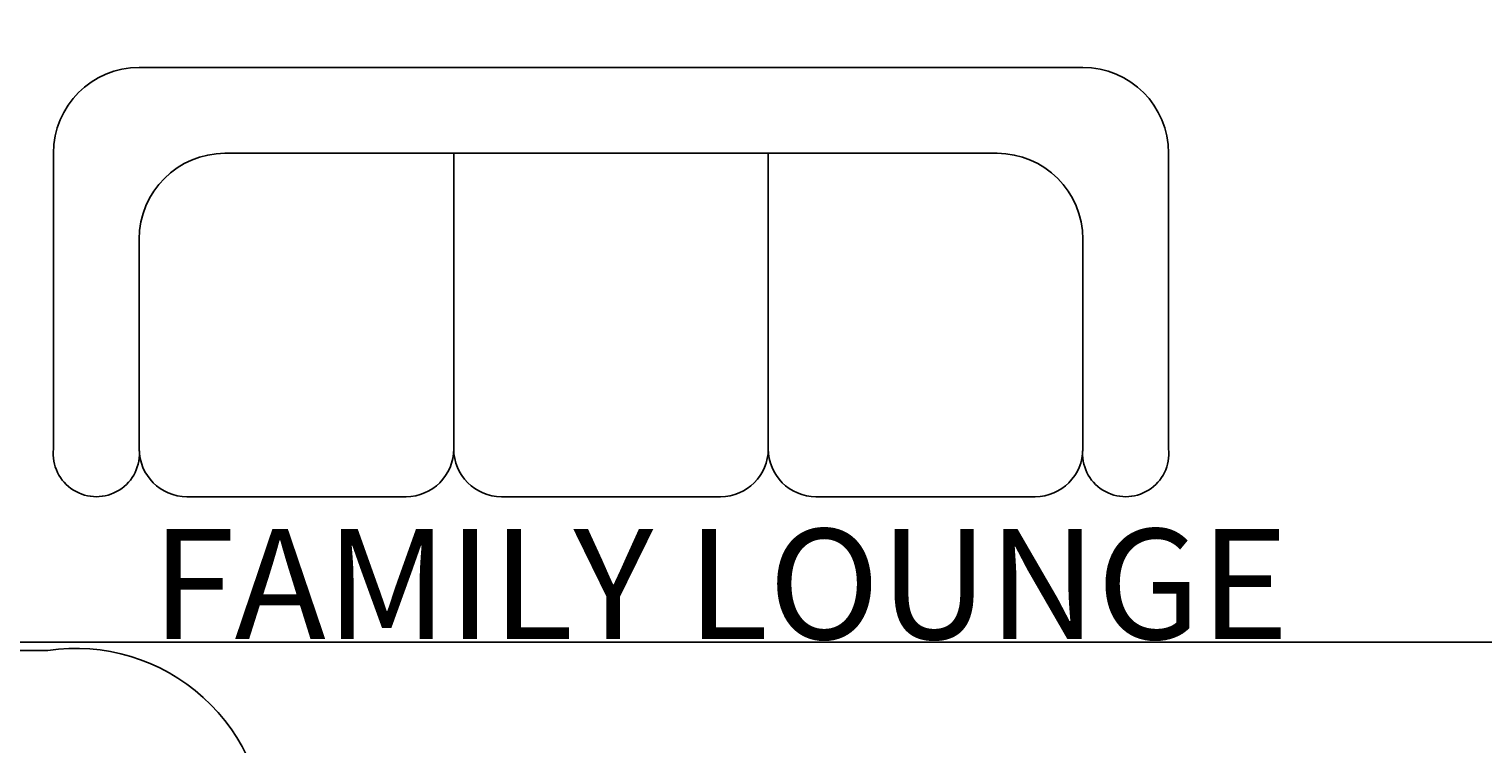
# Model space of a CAD drawing. Units: millimetres. Extents: x 19292 to 100733, y 12374 to 26974.
# Tile 14 of 24: x 28279 to 31036, y 17195 to 18550. Entities that reach past the tile are written whole.
import ezdxf

# ---------------------------------------------------------------- set-up
doc = ezdxf.new("R2010")
doc.units = ezdxf.units.MM
for name, color, linetype, lineweight in [('A-ANNO-DIMS', 2, 'Continuous', 18), ('A-AREA-IDEN', 3, 'Continuous', 25), ('A-FLOR-PATT', 252, 'Continuous', 13), ('A-FURN', 8, 'Continuous', 18)]:
    doc.layers.add(name, color=color, linetype=linetype, lineweight=lineweight)
doc.layers.add('FURNITURE', color=40, linetype='Continuous')
doc.styles.get("Standard").update_dxf_attribs({"font": 'arial.ttf'})
doc.dimstyles.get("Standard").update_dxf_attribs({"dimtxt": 0.18, "dimasz": 0.18, "dimexe": 0.18, "dimexo": 0.0625, "dimgap": 0.09, "dimtad": 0, "dimtih": 1, "dimtoh": 1, "dimdec": 4, "dimzin": 0, "dimdsep": 46, "dimtxsty": 'Standard', "dimcen": 0.09, "dimadec": 0, "dimazin": 0, "dimtfac": 1, "dimtdec": 4, "dimtofl": 0, "dimtmove": 0, "dimatfit": 3, "dimfxl": 1, "dimtolj": 1, "dimtzin": 0, "dimarcsym": 0})

# ---------------------------------------------------------------- blocks, each defined once
blk = doc.blocks.new('3sofa')
at = {"layer": 'FURNITURE'}
for p, q in [((29.7, 0), (-29.7, 0)), ((-35.1, -5.4), (-35.1, -24)), ((24.3, -5.4), (-24.3, -5.4)), ((-9.9, -24), (-9.9, -5.4)), ((9.9, -24), (9.9, -5.4)), ((35.1, -5.4), (35.1, -24)), ((35.1, -5.4), (35.1, -24)), ((-29.7, -10.8), (-29.7, -24)), ((29.7, -10.8), (29.7, -24)), ((-12.9, -27), (-26.7, -27)), ((6.9, -27), (-6.9, -27)), ((26.7, -27), (12.9, -27))]:
    blk.add_line(p, q, dxfattribs=at)
for centre, radius, start, end in [((-29.7, -5.4), 5.4, 90, 180), ((29.7, -5.4), 5.4, 0, 90), ((-24.3, -10.8), 5.4, 90, 180), ((24.3, -10.8), 5.4, 0, 90), ((-32.4, -24.285), 2.715, 173.97442, 6.02558), ((-26.7, -24), 3, 180, 270), ((-12.9, -24), 3, 270, 0), ((-6.9, -24), 3, 180, 270), ((6.9, -24), 3, 270, 0), ((12.9, -24), 3, 180, 270), ((26.7, -24), 3, 270, 0), ((32.4, -24.285), 2.715, 173.97442, 6.02558)]:
    blk.add_arc(centre, radius, start, end, dxfattribs=at)
blk = doc.blocks.new('2sofa-hf')
at = {"layer": 'FURNITURE'}
for p, q in [((-27, -29.849), (-27, 31.724)), ((-21.6, -24.449), (-21.6, 31.724)), ((-21.6, 31.724), (-13.688, 31.724)), ((0, -6.325), (0, 19.345)), ((-21.616, 11.2), (-0.016, 11.2)), ((-21.573, -9.325), (-2.973, -9.325)), ((0, -23.849), (0, -12.325)), ((-16.2, -29.849), (-3, -29.849)), ((-21.6, -35.249), (-2.43, -35.249))]:
    blk.add_line(p, q, dxfattribs=at)
for centre, radius, start, end in [((-24.3, 32.033), 2.718, 353.47896, 186.52104), ((-11.919, 19.923), 11.933, 357.22611, 98.52073), ((-3, -6.325), 3, 270, 0), ((-3, -12.325), 3, 0, 90), ((-16.2, -24.449), 5.4, 180, 270), ((-6, -23.849), 6, 270, 0), ((-21.6, -29.849), 5.4, 180, 270), ((-2.715, -32.549), 2.715, 263.97442, 96.02558)]:
    blk.add_arc(centre, radius, start, end, dxfattribs=at)
blk = doc.blocks.new('*D70')
at = {"layer": 'A-ANNO-DIMS', "color": 0, "lineweight": -2, "transparency": 16777216}
for p, q in [((23573.9, 17387.7), (36879.3, 17387.7)), ((36879.2, 17387.6), (36879.2, 16917.9)), ((36879.2, 16447.9), (36879.2, 16917.6)), ((23573.9, 16447.7), (36879.3, 16447.7))]:
    blk.add_line(p, q, dxfattribs=at)
at = {"layer": 'A-ANNO-DIMS', "color": 0, "transparency": 16777216}
for points in [[(36879.1, 17387.6), (36879.2, 17387.6), (36879.2, 17387.7)], [(36879.1, 16447.9), (36879.2, 16447.9), (36879.2, 16447.7)]]:
    blk.add_solid(points, dxfattribs=at)
at = {"layer": 'Defpoints', "color": 0, "transparency": 16777216}
for p in [(23573.8, 17387.7), (36879.2, 17387.7), (23573.8, 16447.7)]:
    blk.add_point(p, dxfattribs=at)
at = {"layer": 'A-ANNO-DIMS', "color": 0, "transparency": 16777216, "insert": (36879.2, 16917.7), "char_height": 0.18, "attachment_point": 5}
blk.add_mtext('\\A1;940', dxfattribs=at)
blk = doc.blocks.new('*D79')
at = {"layer": 'A-ANNO-DIMS', "color": 0, "lineweight": -2, "transparency": 16777216}
for p, q in [((22694.1, 22860.7), (22694.1, 12808.8)), ((36144.2, 15985.7), (36144.2, 12808.8)), ((22694.3, 12809), (29418.7, 12809)), ((36144, 12809), (29419.6, 12809))]:
    blk.add_line(p, q, dxfattribs=at)
at = {"layer": 'A-ANNO-DIMS', "color": 0, "transparency": 16777216}
for points in [[(22694.3, 12809), (22694.3, 12809), (22694.1, 12809)], [(36144, 12809), (36144, 12809), (36144.2, 12809)]]:
    blk.add_solid(points, dxfattribs=at)
at = {"layer": 'Defpoints', "color": 0, "transparency": 16777216}
for p in [(22694.1, 22860.7), (36144.2, 15985.7), (36144.2, 12809)]:
    blk.add_point(p, dxfattribs=at)
at = {"layer": 'A-ANNO-DIMS', "color": 0, "transparency": 16777216, "insert": (29419.2, 12809), "char_height": 0.18, "attachment_point": 5}
blk.add_mtext('\\A1;13450', dxfattribs=at)
blk = doc.blocks.new('*D82')
at = {"layer": 'A-ANNO-DIMS', "color": 0, "lineweight": -2, "transparency": 16777216}
for p, q in [((27198.8, 13562.8), (27198.8, 23555.9)), ((27199, 23555.7), (29296.4, 23555.7)), ((31394.6, 23555.7), (29297.2, 23555.7)), ((31394.8, 13544.1), (31394.8, 23555.9))]:
    blk.add_line(p, q, dxfattribs=at)
at = {"layer": 'A-ANNO-DIMS', "color": 0, "transparency": 16777216}
for points in [[(27199, 23555.8), (27199, 23555.7), (27198.8, 23555.7)], [(31394.6, 23555.8), (31394.6, 23555.7), (31394.8, 23555.7)]]:
    blk.add_solid(points, dxfattribs=at)
at = {"layer": 'Defpoints', "color": 0, "transparency": 16777216}
for p in [(31394.8, 23555.7), (27198.8, 13562.7), (31394.8, 13544)]:
    blk.add_point(p, dxfattribs=at)
at = {"layer": 'A-ANNO-DIMS', "color": 0, "transparency": 16777216, "insert": (29296.8, 23555.7), "char_height": 0.18, "attachment_point": 5}
blk.add_mtext('\\A1;4196', dxfattribs=at)
blk = doc.blocks.new('*D86')
at = {"layer": 'A-ANNO-DIMS', "color": 0, "lineweight": -2, "transparency": 16777216}
for p, q in [((27198.8, 15132.8), (27198.8, 23555.9)), ((27199, 23555.7), (29198.5, 23555.7)), ((31198.6, 23555.7), (29199.2, 23555.7)), ((31198.8, 15132.8), (31198.8, 23555.9))]:
    blk.add_line(p, q, dxfattribs=at)
at = {"layer": 'A-ANNO-DIMS', "color": 0, "transparency": 16777216}
for points in [[(27199, 23555.8), (27199, 23555.7), (27198.8, 23555.7)], [(31198.6, 23555.8), (31198.6, 23555.7), (31198.8, 23555.7)]]:
    blk.add_solid(points, dxfattribs=at)
at = {"layer": 'Defpoints', "color": 0, "transparency": 16777216}
for p in [(31198.8, 23555.7), (27198.8, 15132.7), (31198.8, 15132.7)]:
    blk.add_point(p, dxfattribs=at)
at = {"layer": 'A-ANNO-DIMS', "color": 0, "transparency": 16777216, "insert": (29198.8, 23555.7), "char_height": 0.18, "attachment_point": 5}
blk.add_mtext('\\A1;4000', dxfattribs=at)

msp = doc.modelspace()

# ---------------------------------------------------------------- hatches: boundary and pattern name
at = {"layer": 'A-FLOR-PATT'}
h = msp.add_hatch(dxfattribs=at)
h.set_pattern_fill('CROSS', color=256, scale=40)
h.paths.add_polyline_path([(36144.169, 19010.725), (33719.169, 19010.725), (33719.169, 18850.725), (33719.169, 18003.026), (33719.169, 15985.725), (36144.169, 15985.725)])
h.paths.add_polyline_path([(36144.132, 22460.725), (34419.132, 22460.725), (34419.132, 22208.026, -0.34415073), (35121.831, 21308.026), (34419.132, 21308.026), (34419.132, 21260.725), (36144.132, 21260.725)])
h.paths.add_polyline_path([(34419.132, 22208.026), (34419.132, 21388.026), (35118.375, 21388.026, 0.32018294)], flags=17)
h.paths.add_polyline_path([(31169.132, 22460.725), (28369.132, 22460.725), (28369.132, 21460.725), (31169.132, 21460.725)])
h.paths.add_polyline_path([(34010.406, 17316.149), (36018.156, 17316.149), (36018.156, 17722.778), (34010.406, 17722.778)], flags=24)
h.paths.add_polyline_path([(34456.896, 21920.301), (35605.434, 21920.301), (35605.434, 22313.518), (34456.896, 22313.518)], flags=25)
h.paths.add_polyline_path([(29263.068, 21823.707), (30421.489, 21823.707), (30421.489, 22034.008), (29263.068, 22034.008)], flags=24)

# ---------------------------------------------------------------- block references
at = {"layer": 'A-FURN', "xscale": 30.13269765108242, "yscale": 30.13269765108242, "zscale": 30.13269765108242}
for name, p in [('3sofa', (29382.472, 18477.205)), ('2sofa-hf', (28726.739, 16416.302))]:
    msp.add_blockref(name, p, dxfattribs=at)

# ---------------------------------------------------------------- texts
at = {"layer": 'A-AREA-IDEN'}
msp.add_text('FAMILY LOUNGE', height=208.87112, dxfattribs=at).set_placement((28511.023, 17393.631))

# ---------------------------------------------------------------- dimensions: what is measured, and where the dimension line sits
at = {"layer": 'A-ANNO-DIMS'}
for base, p1, p2, picture, middle in [((31394.799, 23555.725), (27198.815, 13562.748), (31394.799, 13543.993), '*D82', (29296.807, 23555.725)), ((31198.815, 23555.725), (27198.815, 15132.748), (31198.815, 15132.748), '*D86', (29198.815, 23555.725)), ((36144.169, 12808.993), (22694.132, 22860.725), (36144.169, 15985.725), '*D79', (29419.151, 12808.993))]:
    dim = msp.add_linear_dim(base=base, p1=p1, p2=p2, dimstyle='Standard', override={"dimdec": 0, "dimlfac": 1, "dimrnd": 0, "dimzin": 0, "dimdsep": 46, "dimlunit": 2}, dxfattribs=at)
    dim.commit()
    dim.dimension.update_dxf_attribs({"geometry": picture, "text_midpoint": middle})
dim = msp.add_linear_dim(base=(36879.169, 17387.748), p1=(23573.815, 16447.748), p2=(23573.815, 17387.748), angle=90, dimstyle='Standard', override={"dimdec": 0, "dimlfac": 1, "dimrnd": 0, "dimzin": 0, "dimdsep": 46, "dimlunit": 2}, dxfattribs=at)
dim.commit()
dim.dimension.update_dxf_attribs({"geometry": '*D70', "text_midpoint": (36879.169, 16917.748)})

doc.saveas('drawing.dxf')
